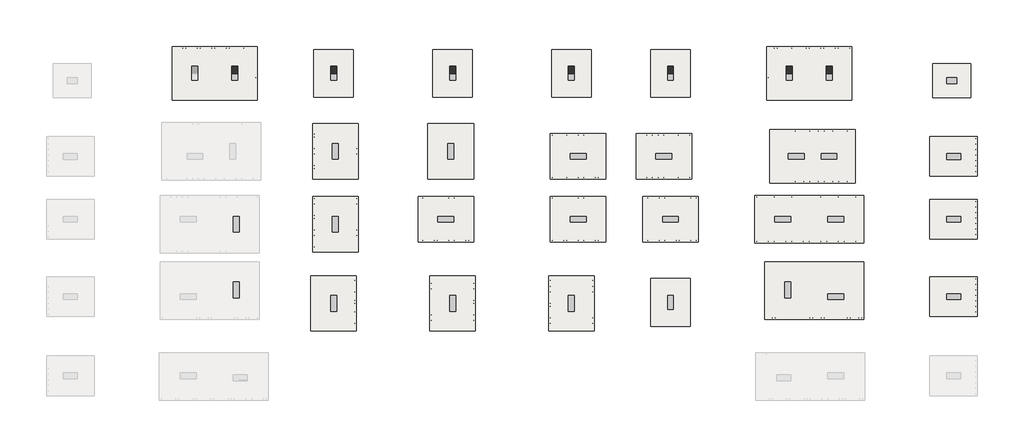
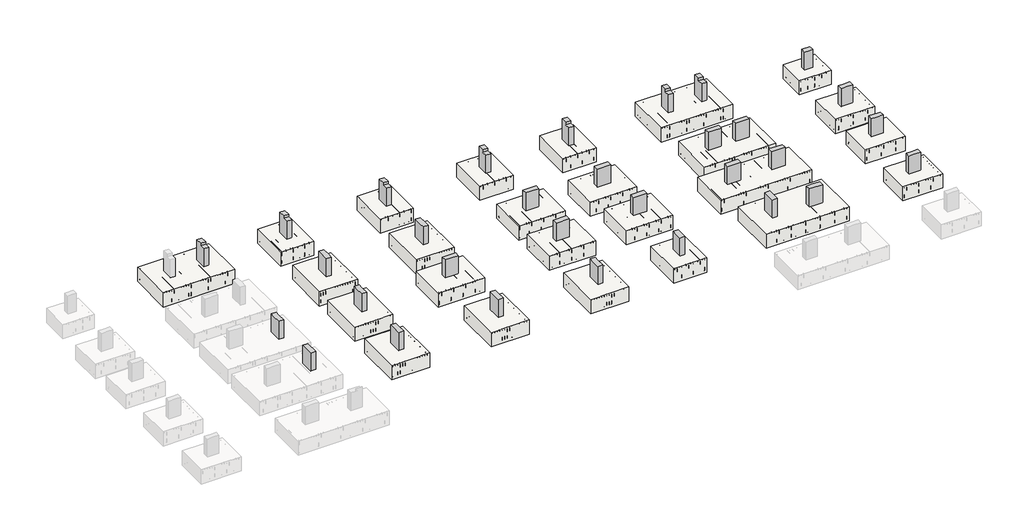
# One storey, part 2 of 21: 31 columns, 25 slabs.
"""IFC4 building model written with IfcOpenShell, lengths in millimetres."""

from ifc_helpers import new_model, si_unit, frame, origin, place, context, project, spatial, polyline, outline, extrude, faceted_brep, transform, mapped, element, save
from components import m_footing_rectangular_1900x1700x900_f1_617558a1, m_footing_rectangular_2300x2800x900_f3_c46bdd4c, m_footing_rectangular_2400x2000x900_f2_ceb4d106, m_footing_rectangular_2700x4300x900_f4_c3563192, m_footing_rectangular_5000x2900x900_f5_2a8e231f, m_footing_rectangular_5500x2400x900_f6_6a8cdcd2

model = new_model("IFC4")

# Units and contexts
model_context = context("Model", 3, world=origin())
ifc_project = project(units=[si_unit("LENGTHUNIT", "METRE", prefix="MILLI")], contexts=[model_context])

# Site, building, storey
site = spatial("IfcSite", under=ifc_project)
building = spatial("IfcBuilding", under=site)
storey = spatial("IfcBuildingStorey", under=building, Elevation=-1100.0)

# Columns
placement = place(None, origin())
element("IfcColumn", 1, ObjectType="M_Concrete-Rectangular-Column : 300X500 C1", at=placement, inside=storey, context=model_context, shape_type="Brep", body=[
    faceted_brep([(20029.1673137, 14604.1704288, -1100.0), (20529.1673137, 14604.1704288, -1100.0), (20529.1673137, 14304.1704288, -1100.0), (20029.1673137, 14304.1704288, -1100.0), (20029.1673137, 14604.1704288, 50.0), (20529.1673137, 14604.1704288, 50.0), (20529.1673137, 14304.1704288, 50.0), (20329.1673137, 14304.1704288, 50.0), (20029.1673137, 14304.1704288, 50.0)], [[[0, 1, 2, 3]], [[1, 0, 4, 5]], [[2, 1, 5, 6]], [[3, 2, 6, 7, 8]], [[0, 3, 8, 4]], [[5, 4, 8, 7, 6]]]),
])
element("IfcColumn", 2, ObjectType="M_Concrete-Rectangular-Column : 300X700 C2", at=placement, inside=storey, context=model_context, shape_type="Brep", body=[
    faceted_brep([(-15760.8326863, 15184.1704288, -1100.0), (-15760.8326863, 14484.1704288, -1100.0), (-16060.8326863, 14484.1704288, -1100.0), (-16060.8326863, 15184.1704288, -1100.0), (-15760.8326863, 15184.1704288, 200.0), (-15760.8326863, 14806.5875097, 200.0), (-15760.8326863, 14806.5875097, 50.0), (-15760.8326863, 14784.1704288, 50.0), (-15760.8326863, 14484.1704288, 50.0), (-15760.8326863, 14484.1704288, -400.0), (-16060.8326863, 14484.1704288, 50.0), (-16060.8326863, 14484.1704288, -400.0), (-16060.8326863, 14784.1704288, 50.0), (-16060.8326863, 14806.5875097, 50.0), (-16060.8326863, 14806.5875097, 200.0), (-16060.8326863, 15184.1704288, 200.0), (-15761.4442233, 14806.5875097, 200.0), (-15761.4442233, 14806.5875097, 50.0)], [[[0, 1, 2, 3]], [[1, 0, 4, 5, 6, 7, 8, 9]], [[2, 1, 9, 8, 10, 11]], [[3, 2, 11, 10, 12, 13, 14, 15]], [[0, 3, 15, 4]], [[4, 15, 14, 16, 5]], [[6, 17, 13, 12, 10, 8, 7]], [[13, 17, 6, 5, 16, 14]]]),
])
element("IfcColumn", 3, ObjectType="M_Concrete-Rectangular-Column : 300X700 C2", at=placement, inside=storey, context=model_context, shape_type="Brep", body=[
    faceted_brep([(-4760.8326863, 15184.1704288, -1100.0), (-4760.8326863, 14484.1704288, -1100.0), (-5060.8326863, 14484.1704288, -1100.0), (-5060.8326863, 15184.1704288, -1100.0), (-4760.8326863, 15184.1704288, 200.0), (-4760.8326863, 14806.5875097, 200.0), (-4760.8326863, 14806.5875097, 50.0), (-4760.8326863, 14784.1704288, 50.0), (-4760.8326863, 14484.1704288, 50.0), (-4760.8326863, 14484.1704288, -400.0), (-5060.8326863, 14484.1704288, 50.0), (-5060.8326863, 14484.1704288, -400.0), (-5060.8326863, 14784.1704288, 50.0), (-5060.8326863, 14806.5875097, 50.0), (-5060.8326863, 14806.5875097, 200.0), (-5060.8326863, 15184.1704288, 200.0)], [[[0, 1, 2, 3]], [[1, 0, 4, 5, 6, 7, 8, 9]], [[2, 1, 9, 8, 10, 11]], [[3, 2, 11, 10, 12, 13, 14, 15]], [[0, 3, 15, 4]], [[4, 15, 14, 5]], [[6, 13, 12, 10, 8, 7]], [[13, 6, 5, 14]]]),
])
element("IfcColumn", 4, ObjectType="M_Concrete-Rectangular-Column : 300X700 C2", at=placement, inside=storey, context=model_context, shape_type="Brep", body=[
    faceted_brep([(1239.1673137, 15184.1704288, -1100.0), (1239.1673137, 14484.1704288, -1100.0), (939.1673137, 14484.1704288, -1100.0), (939.1673137, 15184.1704288, -1100.0), (1239.1673137, 15184.1704288, 200.0), (1239.1673137, 14806.5875097, 200.0), (1239.1673137, 14806.5875097, 50.0), (1239.1673137, 14784.1704288, 50.0), (1239.1673137, 14484.1704288, 50.0), (1239.1673137, 14484.1704288, -400.0), (939.1673137, 14484.1704288, 50.0), (939.1673137, 14484.1704288, -400.0), (939.1673137, 14784.1704288, 50.0), (939.1673137, 14806.5875097, 50.0), (939.1673137, 14806.5875097, 200.0), (939.1673137, 15184.1704288, 200.0)], [[[0, 1, 2, 3]], [[1, 0, 4, 5, 6, 7, 8, 9]], [[2, 1, 9, 8, 10, 11]], [[3, 2, 11, 10, 12, 13, 14, 15]], [[0, 3, 15, 4]], [[4, 15, 14, 5]], [[6, 13, 12, 10, 8, 7]], [[13, 6, 5, 14]]]),
])
element("IfcColumn", 5, ObjectType="M_Concrete-Rectangular-Column : 300X700 C2", at=placement, inside=storey, context=model_context, shape_type="Brep", body=[
    faceted_brep([(6239.1673137, 15184.1301608, -1100.0), (6239.1673137, 14484.1301608, -1100.0), (5939.1673137, 14484.1301608, -1100.0), (5939.1673137, 15184.1301608, -1100.0), (6239.1673137, 15184.1301608, 200.0), (6239.1673137, 14806.5875097, 200.0), (6239.1673137, 14806.5875097, 50.0), (6239.1673137, 14784.1704288, 50.0), (6239.1673137, 14484.1301608, 50.0), (5939.1673137, 14484.1301608, 50.0), (5939.1673137, 14784.1704288, 50.0), (5939.1673137, 14806.5875097, 50.0), (5939.1673137, 14806.5875097, 200.0), (5939.1673137, 15184.1301608, 200.0)], [[[0, 1, 2, 3]], [[1, 0, 4, 5, 6, 7, 8]], [[2, 1, 8, 9]], [[3, 2, 9, 10, 11, 12, 13]], [[0, 3, 13, 4]], [[4, 13, 12, 5]], [[6, 11, 10, 9, 8, 7]], [[11, 6, 5, 12]]]),
])
element("IfcColumn", 6, ObjectType="M_Concrete-Rectangular-Column : 300X700 C2", at=placement, inside=storey, context=model_context, shape_type="Brep", body=[
    faceted_brep([(6239.1673137, 3604.1704288, -1100.0), (6239.1673137, 2904.1704288, -1100.0), (5939.1673137, 2904.1704288, -1100.0), (5939.1673137, 3604.1704288, -1100.0), (6239.1673137, 3604.1704288, 50.0), (6239.1673137, 3276.3054969, 50.0), (6239.1673137, 2904.1704288, 50.0), (5939.1673137, 2904.1704288, 50.0), (5939.1673137, 3304.1704288, 50.0), (5939.1673137, 3604.1704288, 50.0)], [[[0, 1, 2, 3]], [[1, 0, 4, 5, 6]], [[2, 1, 6, 7]], [[3, 2, 7, 8, 9]], [[0, 3, 9, 4]], [[6, 5, 4, 9, 8, 7]]]),
])
element("IfcColumn", 7, ObjectType="M_Concrete-Rectangular-Column : 300X700 C2", at=placement, inside=storey, context=model_context, shape_type="Brep", body=[
    faceted_brep([(12239.1673137, 15184.1704288, -1100.0), (12239.1673137, 14484.1704288, -1100.0), (11939.1673137, 14484.1704288, -1100.0), (11939.1673137, 15184.1704288, -1100.0), (12239.1673137, 15184.1704288, 200.0), (12239.1673137, 14806.5875097, 200.0), (12239.1673137, 14806.5875097, 50.0), (12239.1673137, 14784.1704288, 50.0), (12239.1673137, 14484.1704288, 50.0), (12239.1673137, 14484.1704288, -400.0), (11939.1673137, 14484.1704288, 50.0), (11939.1673137, 14484.1704288, -400.0), (11939.1673137, 14784.1704288, 50.0), (11939.1673137, 14806.5875097, 50.0), (11939.1673137, 14806.5875097, 200.0), (11939.1673137, 15184.1704288, 200.0)], [[[0, 1, 2, 3]], [[1, 0, 4, 5, 6, 7, 8, 9]], [[2, 1, 9, 8, 10, 11]], [[3, 2, 11, 10, 12, 13, 14, 15]], [[0, 3, 15, 4]], [[4, 15, 14, 5]], [[6, 13, 12, 10, 8, 7]], [[13, 6, 5, 14]]]),
])
element("IfcColumn", 8, ObjectType="M_Concrete-Rectangular-Column : 300X700 C2", at=placement, inside=storey, context=model_context, shape_type="SweptSolid", body=[
    extrude(outline(polyline([(15184.1704288, -1100.0), (14484.1704288, -1100.0), (14484.1704288, 50.0), (14806.5875097, 50.0), (14806.5875097, 200.0), (15184.1704288, 200.0), (15184.1704288, -1100.0)])), frame((13939.1673137, 0.0, 0.0), z_axis=(1.0, 0.0, 0.0), x_axis=(0.0, 1.0, 0.0)), (0.0, 0.0, 1.0), 300.0),
])
element("IfcColumn", 9, ObjectType="M_Concrete-Rectangular-Column : 300X700 C2", at=placement, inside=storey, context=model_context, shape_type="Brep", body=[
    faceted_brep([(20029.1673137, 10779.2254822, -1100.0), (20729.1673137, 10779.2254822, -1100.0), (20729.1673137, 10479.2254822, -1100.0), (20029.1673137, 10479.2254822, -1100.0), (20029.1673137, 10779.2254822, -400.0), (20029.1673137, 10779.2254822, 50.0), (20329.1673137, 10779.2254822, 50.0), (20729.1673137, 10779.2254822, 50.0), (20729.1673137, 10479.2254822, 50.0), (20329.1673137, 10479.2254822, 50.0), (20029.1673137, 10479.2254822, 50.0), (20029.1673137, 10479.2254822, -400.0)], [[[0, 1, 2, 3]], [[1, 0, 4, 5, 6, 7]], [[2, 1, 7, 8]], [[3, 2, 8, 9, 10, 11]], [[0, 3, 11, 10, 5, 4]], [[7, 6, 5, 10, 9, 8]]]),
])
element("IfcColumn", 10, ObjectType="M_Concrete-Rectangular-Column : 300X700 C2", at=placement, inside=storey, context=model_context, shape_type="Brep", body=[
    faceted_brep([(20029.1673137, 7604.1704288, -1100.0), (20729.1673137, 7604.1704288, -1100.0), (20729.1673137, 7304.1704288, -1100.0), (20029.1673137, 7304.1704288, -1100.0), (20029.1673137, 7604.1704288, -400.0), (20029.1673137, 7604.1704288, 50.0), (20329.1673137, 7604.1704288, 50.0), (20729.1673137, 7604.1704288, 50.0), (20729.1673137, 7304.1704288, 50.0), (20329.1673137, 7304.1704288, 50.0), (20029.1673137, 7304.1704288, 50.0), (20029.1673137, 7304.1704288, -400.0)], [[[0, 1, 2, 3]], [[1, 0, 4, 5, 6, 7]], [[2, 1, 7, 8]], [[3, 2, 8, 9, 10, 11]], [[0, 3, 11, 10, 5, 4]], [[7, 6, 5, 10, 9, 8]]]),
])
element("IfcColumn", 11, ObjectType="M_Concrete-Rectangular-Column : 300X700 C2", at=placement, inside=storey, context=model_context, shape_type="Brep", body=[
    faceted_brep([(20029.1673137, 3694.1704288, -1100.0), (20729.1673137, 3694.1704288, -1100.0), (20729.1673137, 3394.1704288, -1100.0), (20029.1673137, 3394.1704288, -1100.0), (20029.1673137, 3694.1704288, -400.0), (20029.1673137, 3694.1704288, 50.0), (20329.1673137, 3694.1704288, 50.0), (20729.1673137, 3694.1704288, 50.0), (20729.1673137, 3394.1704288, 50.0), (20329.1673137, 3394.1704288, 50.0), (20029.1673137, 3394.1704288, 50.0), (20029.1673137, 3394.1704288, -400.0)], [[[0, 1, 2, 3]], [[1, 0, 4, 5, 6, 7]], [[2, 1, 7, 8]], [[3, 2, 8, 9, 10, 11]], [[0, 3, 11, 10, 5, 4]], [[7, 6, 5, 10, 9, 8]]]),
])
element("IfcColumn", 12, ObjectType="M_Concrete-Rectangular-Column : 300X700 C2", at=placement, inside=storey, context=model_context, shape_type="Brep", body=[
    faceted_brep([(-11060.8326863, 14484.1704288, -1100.0), (-11060.8326863, 15184.1704288, -1100.0), (-10760.8326863, 15184.1704288, -1100.0), (-10760.8326863, 14484.1704288, -1100.0), (-11060.8326863, 14484.1704288, -400.0), (-11060.8326863, 14484.1704288, 50.0), (-11060.8326863, 14784.1704288, 50.0), (-11060.8326863, 14806.5875097, 50.0), (-11060.8326863, 14806.5875097, 200.0), (-11060.8326863, 15184.1704288, 200.0), (-10760.8326863, 15184.1704288, 200.0), (-10760.8326863, 14806.5875097, 200.0), (-10760.8326863, 14806.5875097, 50.0), (-10760.8326863, 14784.1704288, 50.0), (-10760.8326863, 14484.1704288, 50.0), (-10760.8326863, 14484.1704288, -400.0)], [[[0, 1, 2, 3]], [[1, 0, 4, 5, 6, 7, 8, 9]], [[2, 1, 9, 10]], [[3, 2, 10, 11, 12, 13, 14, 15]], [[0, 3, 15, 14, 5, 4]], [[10, 9, 8, 11]], [[12, 7, 6, 5, 14, 13]], [[7, 12, 11, 8]]]),
])
element("IfcColumn", 13, ObjectType="M_Concrete-Rectangular-Column : 300X800 C3", at=placement, inside=storey, context=model_context, shape_type="Brep", body=[
    faceted_brep([(-15970.8326863, 6804.1704288, -1100.0), (-15970.8326863, 7604.1704288, -1100.0), (-15670.8326863, 7604.1704288, -1100.0), (-15670.8326863, 6804.1704288, -1100.0), (-15970.8326863, 6804.1704288, 50.0), (-15970.8326863, 7304.1704288, 50.0), (-15970.8326863, 7354.7105431, 50.0), (-15970.8326863, 7604.1704288, 50.0), (-15670.8326863, 7604.1704288, 50.0), (-15670.8326863, 7604.1704288, -400.0), (-15670.8326863, 7304.1704288, 50.0), (-15670.8326863, 6804.1704288, 50.0)], [[[0, 1, 2, 3]], [[1, 0, 4, 5, 6, 7]], [[2, 1, 7, 8, 9]], [[3, 2, 9, 8, 10, 11]], [[0, 3, 11, 4]], [[7, 6, 5, 4, 11, 10, 8]]]),
])
element("IfcColumn", 14, ObjectType="M_Concrete-Rectangular-Column : 300X800 C3", at=placement, inside=storey, context=model_context, shape_type="SweptSolid", body=[
    extrude(outline(polyline([(-15970.8326863, 3484.1704288), (-15970.8326863, 4284.1704288), (-15670.8326863, 4284.1704288), (-15670.8326863, 3484.1704288), (-15970.8326863, 3484.1704288)])), frame((0.0, 0.0, -1100.0), z_axis=(0.0, 0.0, 1.0), x_axis=(1.0, 0.0, 0.0)), (0.0, 0.0, 1.0), 1150.0),
])
element("IfcColumn", 15, ObjectType="M_Concrete-Rectangular-Column : 300X800 C3", at=placement, inside=storey, context=model_context, shape_type="Brep", body=[
    faceted_brep([(-10670.8326863, 11284.1704288, -1100.0), (-10670.8326863, 10484.1704288, -1100.0), (-10970.8326863, 10484.1704288, -1100.0), (-10970.8326863, 11284.1704288, -1100.0), (-10670.8326863, 11284.1704288, 50.0), (-10670.8326863, 10784.1704288, 50.0), (-10670.8326863, 10484.1704288, 50.0), (-10670.8326863, 10484.1704288, -400.0), (-10970.8326863, 10484.1704288, 50.0), (-10970.8326863, 10484.1704288, -400.0), (-10970.8326863, 10784.1704288, 50.0), (-10970.8326863, 11284.1704288, 50.0)], [[[0, 1, 2, 3]], [[1, 0, 4, 5, 6, 7]], [[2, 1, 7, 6, 8, 9]], [[3, 2, 9, 8, 10, 11]], [[0, 3, 11, 4]], [[6, 5, 4, 11, 10, 8]]]),
])
element("IfcColumn", 16, ObjectType="M_Concrete-Rectangular-Column : 300X800 C3", at=placement, inside=storey, context=model_context, shape_type="Brep", body=[
    faceted_brep([(-10670.8326863, 7604.1704288, -1100.0), (-10670.8326863, 6804.1704288, -1100.0), (-10970.8326863, 6804.1704288, -1100.0), (-10970.8326863, 7604.1704288, -1100.0), (-10670.8326863, 7604.1704288, -400.0), (-10670.8326863, 7604.1704288, 50.0), (-10670.8326863, 7350.6221749, 50.0), (-10670.8326863, 6804.1704288, 50.0), (-10970.8326863, 6804.1704288, 50.0), (-10970.8326863, 7304.1704288, 50.0), (-10970.8326863, 7604.1704288, 50.0), (-10970.8326863, 7604.1704288, -400.0)], [[[0, 1, 2, 3]], [[1, 0, 4, 5, 6, 7]], [[2, 1, 7, 8]], [[3, 2, 8, 9, 10, 11]], [[0, 3, 11, 10, 5, 4]], [[7, 6, 5, 10, 9, 8]]]),
])
element("IfcColumn", 17, ObjectType="M_Concrete-Rectangular-Column : 300X800 C3", at=placement, inside=storey, context=model_context, shape_type="Brep", body=[
    faceted_brep([(-4850.8326863, 11284.1704288, -1100.0), (-4850.8326863, 10484.1704288, -1100.0), (-5150.8326863, 10484.1704288, -1100.0), (-5150.8326863, 11284.1704288, -1100.0), (-4850.8326863, 11284.1704288, 50.0), (-4850.8326863, 10784.1704288, 50.0), (-4850.8326863, 10484.1704288, 50.0), (-4850.8326863, 10484.1704288, -400.0), (-5150.8326863, 10484.1704288, 50.0), (-5150.8326863, 10484.1704288, -400.0), (-5150.8326863, 10784.1704288, 50.0), (-5150.8326863, 11284.1704288, 50.0)], [[[0, 1, 2, 3]], [[1, 0, 4, 5, 6, 7]], [[2, 1, 7, 6, 8, 9]], [[3, 2, 9, 8, 10, 11]], [[0, 3, 11, 4]], [[6, 5, 4, 11, 10, 8]]]),
])
element("IfcColumn", 18, ObjectType="M_Concrete-Rectangular-Column : 300X800 C3", at=placement, inside=storey, context=model_context, shape_type="Brep", body=[
    faceted_brep([(-10760.8326863, 3604.1704288, -1100.0), (-10760.8326863, 2804.1704288, -1100.0), (-11060.8326863, 2804.1704288, -1100.0), (-11060.8326863, 3604.1704288, -1100.0), (-10760.8326863, 3604.1704288, 50.0), (-10760.8326863, 3304.1704288, 50.0), (-10760.8326863, 2804.1704288, 50.0), (-11060.8326863, 2804.1704288, 50.0), (-11060.8326863, 3303.9418326, 50.0), (-11060.8326863, 3604.1704288, 50.0)], [[[0, 1, 2, 3]], [[1, 0, 4, 5, 6]], [[2, 1, 6, 7]], [[3, 2, 7, 8, 9]], [[0, 3, 9, 4]], [[6, 5, 4, 9, 8, 7]]]),
])
element("IfcColumn", 19, ObjectType="M_Concrete-Rectangular-Column : 300X800 C3", at=placement, inside=storey, context=model_context, shape_type="Brep", body=[
    faceted_brep([(-4760.8326863, 3604.1704288, -1100.0), (-4760.8326863, 2804.1704288, -1100.0), (-5060.8326863, 2804.1704288, -1100.0), (-5060.8326863, 3604.1704288, -1100.0), (-4760.8326863, 3604.1704288, -400.0), (-4760.8326863, 3604.1704288, 50.0), (-4760.8326863, 3304.1704288, 50.0), (-4760.8326863, 2804.1704288, 50.0), (-5060.8326863, 2804.1704288, 50.0), (-5060.8326863, 3304.1704288, 50.0), (-5060.8326863, 3604.1704288, 50.0), (-5060.8326863, 3604.1704288, -400.0)], [[[0, 1, 2, 3]], [[1, 0, 4, 5, 6, 7]], [[2, 1, 7, 8]], [[3, 2, 8, 9, 10, 11]], [[0, 3, 11, 10, 5, 4]], [[7, 6, 5, 10, 9, 8]]]),
])
element("IfcColumn", 20, ObjectType="M_Concrete-Rectangular-Column : 300X800 C3", at=placement, inside=storey, context=model_context, shape_type="Brep", body=[
    faceted_brep([(-5650.8326863, 7604.1704288, -1100.0), (-4850.8326863, 7604.1704288, -1100.0), (-4850.8326863, 7304.1704288, -1100.0), (-5650.8326863, 7304.1704288, -1100.0), (-5650.8326863, 7604.1704288, -400.0), (-5650.8326863, 7604.1704288, 50.0), (-4850.8326863, 7604.1704288, 50.0), (-4850.8326863, 7604.1704288, -400.0), (-4850.8326863, 7304.1704288, 50.0), (-4850.8326863, 7304.1704288, -400.0), (-5650.8326863, 7304.1704288, 50.0), (-5650.8326863, 7304.1704288, -400.0)], [[[0, 1, 2, 3]], [[1, 0, 4, 5, 6, 7]], [[2, 1, 7, 6, 8, 9]], [[3, 2, 9, 8, 10, 11]], [[0, 3, 11, 10, 5, 4]], [[6, 5, 10, 8]]]),
])
element("IfcColumn", 21, ObjectType="M_Concrete-Rectangular-Column : 300X800 C3", at=placement, inside=storey, context=model_context, shape_type="Brep", body=[
    faceted_brep([(1029.1673137, 10784.1704288, -1100.0), (1829.1673137, 10784.1704288, -1100.0), (1829.1673137, 10484.1704288, -1100.0), (1029.1673137, 10484.1704288, -1100.0), (1029.1673137, 10784.1704288, -400.0), (1029.1673137, 10784.1704288, 50.0), (1829.1673137, 10784.1704288, 50.0), (1829.1673137, 10784.1704288, -400.0), (1829.1673137, 10484.1704288, 50.0), (1829.1673137, 10484.1704288, -400.0), (1029.1673137, 10484.1704288, 50.0), (1029.1673137, 10484.1704288, -400.0)], [[[0, 1, 2, 3]], [[1, 0, 4, 5, 6, 7]], [[2, 1, 7, 6, 8, 9]], [[3, 2, 9, 8, 10, 11]], [[0, 3, 11, 10, 5, 4]], [[6, 5, 10, 8]]]),
])
element("IfcColumn", 22, ObjectType="M_Concrete-Rectangular-Column : 300X800 C3", at=placement, inside=storey, context=model_context, shape_type="Brep", body=[
    faceted_brep([(5349.1673137, 10784.1704288, -1100.0), (6149.1673137, 10784.1704288, -1100.0), (6149.1673137, 10484.1704288, -1100.0), (5349.1673137, 10484.1704288, -1100.0), (5349.1673137, 10784.1704288, -400.0), (5349.1673137, 10784.1704288, 50.0), (6149.1673137, 10784.1704288, 50.0), (6149.1673137, 10784.1704288, -400.0), (6149.1673137, 10634.1704288, 50.0), (6149.1673137, 10484.1704288, 50.0), (5349.1673137, 10484.1704288, 50.0), (5349.1673137, 10484.1704288, -400.0)], [[[0, 1, 2, 3]], [[1, 0, 4, 5, 6, 7]], [[2, 1, 7, 6, 8, 9]], [[3, 2, 9, 10, 11]], [[0, 3, 11, 10, 5, 4]], [[6, 5, 10, 9, 8]]]),
])
element("IfcColumn", 23, ObjectType="M_Concrete-Rectangular-Column : 300X800 C3", at=placement, inside=storey, context=model_context, shape_type="Brep", body=[
    faceted_brep([(5689.1673137, 7604.1704288, -1100.0), (6489.1673137, 7604.1704288, -1100.0), (6489.1673137, 7304.1704288, -1100.0), (5689.1673137, 7304.1704288, -1100.0), (5689.1673137, 7604.1704288, -400.0), (5689.1673137, 7604.1704288, 50.0), (6489.1673137, 7604.1704288, 50.0), (6489.1673137, 7604.1704288, -400.0), (6489.1673137, 7304.1704288, 50.0), (6489.1673137, 7304.1704288, -400.0), (5689.1673137, 7304.1704288, 50.0), (5689.1673137, 7304.1704288, -400.0)], [[[0, 1, 2, 3]], [[1, 0, 4, 5, 6, 7]], [[2, 1, 7, 6, 8, 9]], [[3, 2, 9, 8, 10, 11]], [[0, 3, 11, 10, 5, 4]], [[6, 5, 10, 8]]]),
])
element("IfcColumn", 24, ObjectType="M_Concrete-Rectangular-Column : 300X800 C3", at=placement, inside=storey, context=model_context, shape_type="Brep", body=[
    faceted_brep([(1029.1673137, 7604.1704288, -1100.0), (1829.1673137, 7604.1704288, -1100.0), (1829.1673137, 7304.1704288, -1100.0), (1029.1673137, 7304.1704288, -1100.0), (1029.1673137, 7604.1704288, 50.0), (1829.1673137, 7604.1704288, 50.0), (1829.1673137, 7604.1704288, -400.0), (1829.1673137, 7304.1704288, 50.0), (1829.1673137, 7304.1704288, -400.0), (1029.1673137, 7304.1704288, 50.0)], [[[0, 1, 2, 3]], [[1, 0, 4, 5, 6]], [[2, 1, 6, 5, 7, 8]], [[3, 2, 8, 7, 9]], [[0, 3, 9, 4]], [[5, 4, 9, 7]]]),
])
element("IfcColumn", 25, ObjectType="M_Concrete-Rectangular-Column : 300X800 C3", at=placement, inside=storey, context=model_context, shape_type="Brep", body=[
    faceted_brep([(939.1673137, 2804.1704288, -1100.0), (939.1673137, 3604.1704288, -1100.0), (1239.1673137, 3604.1704288, -1100.0), (1239.1673137, 2804.1704288, -1100.0), (939.1673137, 2804.1704288, 50.0), (939.1673137, 3304.1704288, 50.0), (939.1673137, 3604.1704288, 50.0), (939.1673137, 3604.1704288, -400.0), (1239.1673137, 3604.1704288, 50.0), (1239.1673137, 3604.1704288, -400.0), (1239.1673137, 3304.1704288, 50.0), (1239.1673137, 2804.1704288, 50.0)], [[[0, 1, 2, 3]], [[1, 0, 4, 5, 6, 7]], [[2, 1, 7, 6, 8, 9]], [[3, 2, 9, 8, 10, 11]], [[0, 3, 11, 4]], [[6, 5, 4, 11, 10, 8]]]),
])
element("IfcColumn", 26, ObjectType="M_Concrete-Rectangular-Column : 300X800 C3", at=placement, inside=storey, context=model_context, shape_type="Brep", body=[
    faceted_brep([(13689.1673137, 10784.1704288, -1100.0), (14489.1673137, 10784.1704288, -1100.0), (14489.1673137, 10484.1704288, -1100.0), (13689.1673137, 10484.1704288, -1100.0), (13689.1673137, 10784.1704288, -400.0), (13689.1673137, 10784.1704288, 50.0), (14489.1673137, 10784.1704288, 50.0), (14489.1673137, 10784.1704288, -400.0), (14489.1673137, 10484.1704288, 50.0), (14489.1673137, 10484.1704288, -400.0), (13689.1673137, 10484.1704288, 50.0), (13689.1673137, 10484.1704288, -400.0)], [[[0, 1, 2, 3]], [[1, 0, 4, 5, 6, 7]], [[2, 1, 7, 6, 8, 9]], [[3, 2, 9, 8, 10, 11]], [[0, 3, 11, 10, 5, 4]], [[6, 5, 10, 8]]]),
])
element("IfcColumn", 27, ObjectType="M_Concrete-Rectangular-Column : 300X800 C3", at=placement, inside=storey, context=model_context, shape_type="Brep", body=[
    faceted_brep([(12029.1673137, 10784.1704288, -1100.0), (12829.1673137, 10784.1704288, -1100.0), (12829.1673137, 10484.1704288, -1100.0), (12029.1673137, 10484.1704288, -1100.0), (12029.1673137, 10784.1704288, -400.0), (12029.1673137, 10784.1704288, 50.0), (12829.1673137, 10784.1704288, 50.0), (12829.1673137, 10784.1704288, -400.0), (12829.1673137, 10484.1704288, 50.0), (12829.1673137, 10484.1704288, -400.0), (12029.1673137, 10484.1704288, 50.0), (12029.1673137, 10484.1704288, -400.0)], [[[0, 1, 2, 3]], [[1, 0, 4, 5, 6, 7]], [[2, 1, 7, 6, 8, 9]], [[3, 2, 9, 8, 10, 11]], [[0, 3, 11, 10, 5, 4]], [[6, 5, 10, 8]]]),
])
element("IfcColumn", 28, ObjectType="M_Concrete-Rectangular-Column : 300X800 C3", at=placement, inside=storey, context=model_context, shape_type="Brep", body=[
    faceted_brep([(11349.1673137, 7604.1704288, -1100.0), (12149.1673137, 7604.1704288, -1100.0), (12149.1673137, 7304.1704288, -1100.0), (11349.1673137, 7304.1704288, -1100.0), (11349.1673137, 7604.1704288, -400.0), (11349.1673137, 7604.1704288, 50.0), (12149.1673137, 7604.1704288, 50.0), (12149.1673137, 7604.1704288, -400.0), (12149.1673137, 7304.1704288, 50.0), (12149.1673137, 7304.1704288, -400.0), (11349.1673137, 7304.1704288, 50.0), (11349.1673137, 7304.1704288, -400.0)], [[[0, 1, 2, 3]], [[1, 0, 4, 5, 6, 7]], [[2, 1, 7, 6, 8, 9]], [[3, 2, 9, 8, 10, 11]], [[0, 3, 11, 10, 5, 4]], [[6, 5, 10, 8]]]),
])
element("IfcColumn", 29, ObjectType="M_Concrete-Rectangular-Column : 300X800 C3", at=placement, inside=storey, context=model_context, shape_type="Brep", body=[
    faceted_brep([(14029.1673137, 7604.1704288, -1100.0), (14829.1673137, 7604.1704288, -1100.0), (14829.1673137, 7304.1704288, -1100.0), (14029.1673137, 7304.1704288, -1100.0), (14029.1673137, 7604.1704288, -400.0), (14029.1673137, 7604.1704288, 50.0), (14829.1673137, 7604.1704288, 50.0), (14829.1673137, 7604.1704288, -400.0), (14829.1673137, 7304.1704288, 50.0), (14829.1673137, 7304.1704288, -400.0), (14029.1673137, 7304.1704288, 50.0), (14029.1673137, 7304.1704288, -400.0)], [[[0, 1, 2, 3]], [[1, 0, 4, 5, 6, 7]], [[2, 1, 7, 6, 8, 9]], [[3, 2, 9, 8, 10, 11]], [[0, 3, 11, 10, 5, 4]], [[6, 5, 10, 8]]]),
])
element("IfcColumn", 30, ObjectType="M_Concrete-Rectangular-Column : 300X800 C3", at=placement, inside=storey, context=model_context, shape_type="Brep", body=[
    faceted_brep([(14029.1673137, 3694.1704288, -1100.0), (14829.1673137, 3694.1704288, -1100.0), (14829.1673137, 3394.1704288, -1100.0), (14029.1673137, 3394.1704288, -1100.0), (14029.1673137, 3694.1704288, -400.0), (14029.1673137, 3694.1704288, 50.0), (14329.1673137, 3694.1704288, 50.0), (14829.1673137, 3694.1704288, 50.0), (14829.1673137, 3394.1704288, 50.0), (14329.1673137, 3394.1704288, 50.0), (14029.1673137, 3394.1704288, 50.0), (14029.1673137, 3394.1704288, -400.0)], [[[0, 1, 2, 3]], [[1, 0, 4, 5, 6, 7]], [[2, 1, 7, 8]], [[3, 2, 8, 9, 10, 11]], [[0, 3, 11, 10, 5, 4]], [[7, 6, 5, 10, 9, 8]]]),
])
element("IfcColumn", 31, ObjectType="M_Concrete-Rectangular-Column : 300X800 C3", at=placement, inside=storey, context=model_context, shape_type="SweptSolid", body=[
    extrude(outline(polyline([(11849.1673137, 3484.1704288), (11849.1673137, 4284.1704288), (12149.1673137, 4284.1704288), (12149.1673137, 3484.1704288), (11849.1673137, 3484.1704288)])), frame((0.0, 0.0, -1100.0), z_axis=(0.0, 0.0, 1.0), x_axis=(1.0, 0.0, 0.0)), (0.0, 0.0, 1.0), 1150.0),
])

# Slabs
m_footing_rectangular_1900x1700x900_f1_shape = m_footing_rectangular_1900x1700x900_f1_617558a1(model_context)
element("IfcSlab", 32, ObjectType="M_Footing-Rectangular : 1900X1700X900 F1", at=placement, inside=storey, context=model_context, shape_type="MappedRepresentation", body=[
    mapped(m_footing_rectangular_1900x1700x900_f1_shape, transform((20279.1673137, 14454.1704288, -1100.0), x_axis=(1.0, 0.0, 0.0), y_axis=(0.0, 1.0, 0.0), z_axis=(0.0, 0.0, 1.0))),
])
m_footing_rectangular_2300x2800x900_f3_shape = m_footing_rectangular_2300x2800x900_f3_c46bdd4c(model_context)
element("IfcSlab", 33, ObjectType="M_Footing-Rectangular : 2300X2800X900 F3", at=placement, inside=storey, context=model_context, shape_type="MappedRepresentation", body=[
    mapped(m_footing_rectangular_2300x2800x900_f3_shape, transform((-10820.8326863, 10884.1704288, -1100.0), x_axis=(1.0, 0.0, 0.0), y_axis=(0.0, 1.0, 0.0), z_axis=(0.0, 0.0, 1.0))),
])
element("IfcSlab", 34, ObjectType="M_Footing-Rectangular : 2300X2800X900 F3", at=placement, inside=storey, context=model_context, shape_type="MappedRepresentation", body=[
    mapped(m_footing_rectangular_2300x2800x900_f3_shape, transform((-5000.8326863, 10884.1704288, -1100.0), x_axis=(1.0, 0.0, 0.0), y_axis=(0.0, 1.0, 0.0), z_axis=(0.0, 0.0, 1.0))),
])
element("IfcSlab", 35, ObjectType="M_Footing-Rectangular : 2300X2800X900 F3", at=placement, inside=storey, context=model_context, shape_type="MappedRepresentation", body=[
    mapped(m_footing_rectangular_2300x2800x900_f3_shape, transform((-10820.8326863, 7204.1704288, -1100.0), x_axis=(1.0, 0.0, 0.0), y_axis=(0.0, 1.0, 0.0), z_axis=(0.0, 0.0, 1.0))),
])
element("IfcSlab", 36, ObjectType="M_Footing-Rectangular : 2300X2800X900 F3", at=placement, inside=storey, context=model_context, shape_type="MappedRepresentation", body=[
    mapped(m_footing_rectangular_2300x2800x900_f3_shape, transform((-10910.8326863, 3204.1704288, -1100.0), x_axis=(1.0, 0.0, 0.0), y_axis=(0.0, 1.0, 0.0), z_axis=(0.0, 0.0, 1.0))),
])
element("IfcSlab", 37, ObjectType="M_Footing-Rectangular : 2300X2800X900 F3", at=placement, inside=storey, context=model_context, shape_type="MappedRepresentation", body=[
    mapped(m_footing_rectangular_2300x2800x900_f3_shape, transform((-4910.8326863, 3204.1704288, -1100.0), x_axis=(1.0, 0.0, 0.0), y_axis=(0.0, 1.0, 0.0), z_axis=(0.0, 0.0, 1.0))),
])
element("IfcSlab", 38, ObjectType="M_Footing-Rectangular : 2300X2800X900 F3", at=placement, inside=storey, context=model_context, shape_type="MappedRepresentation", body=[
    mapped(m_footing_rectangular_2300x2800x900_f3_shape, transform((-5250.8326863, 7454.1704288, -1100.0), x_axis=(0.0, 1.0, 0.0), y_axis=(-1.0, 0.0, 0.0), z_axis=(0.0, 0.0, 1.0))),
])
element("IfcSlab", 39, ObjectType="M_Footing-Rectangular : 2300X2800X900 F3", at=placement, inside=storey, context=model_context, shape_type="MappedRepresentation", body=[
    mapped(m_footing_rectangular_2300x2800x900_f3_shape, transform((1429.1673137, 10634.1704288, -1100.0), x_axis=(0.0, 1.0, 0.0), y_axis=(-1.0, 0.0, 0.0), z_axis=(0.0, 0.0, 1.0))),
])
element("IfcSlab", 40, ObjectType="M_Footing-Rectangular : 2300X2800X900 F3", at=placement, inside=storey, context=model_context, shape_type="MappedRepresentation", body=[
    mapped(m_footing_rectangular_2300x2800x900_f3_shape, transform((1429.1673137, 7454.1704288, -1100.0), x_axis=(0.0, 1.0, 0.0), y_axis=(-1.0, 0.0, 0.0), z_axis=(0.0, 0.0, 1.0))),
])
element("IfcSlab", 41, ObjectType="M_Footing-Rectangular : 2300X2800X900 F3", at=placement, inside=storey, context=model_context, shape_type="MappedRepresentation", body=[
    mapped(m_footing_rectangular_2300x2800x900_f3_shape, transform((1089.1673137, 3204.1704288, -1100.0), x_axis=(-1.0, 0.0, 0.0), y_axis=(0.0, -1.0, 0.0), z_axis=(0.0, 0.0, 1.0))),
])
element("IfcSlab", 42, ObjectType="M_Footing-Rectangular : 2300X2800X900 F3", at=placement, inside=storey, context=model_context, shape_type="MappedRepresentation", body=[
    mapped(m_footing_rectangular_2300x2800x900_f3_shape, transform((6089.1673137, 7454.1704288, -1100.0), x_axis=(0.0, -1.0, 0.0), y_axis=(1.0, 0.0, 0.0), z_axis=(0.0, 0.0, 1.0))),
])
element("IfcSlab", 43, ObjectType="M_Footing-Rectangular : 2300X2800X900 F3", at=placement, inside=storey, context=model_context, shape_type="MappedRepresentation", body=[
    mapped(m_footing_rectangular_2300x2800x900_f3_shape, transform((5749.1673137, 10634.1704288, -1100.0), x_axis=(0.0, -1.0, 0.0), y_axis=(1.0, 0.0, 0.0), z_axis=(0.0, 0.0, 1.0))),
])
m_footing_rectangular_2400x2000x900_f2_shape = m_footing_rectangular_2400x2000x900_f2_ceb4d106(model_context)
element("IfcSlab", 44, ObjectType="M_Footing-Rectangular : 2400X2000X900 F2", at=placement, inside=storey, context=model_context, shape_type="MappedRepresentation", body=[
    mapped(m_footing_rectangular_2400x2000x900_f2_shape, transform((-10910.8326863, 14834.170481, -1100.0), x_axis=(0.0, 1.0, 0.0), y_axis=(-1.0, 0.0, 0.0), z_axis=(0.0, 0.0, 1.0))),
])
element("IfcSlab", 45, ObjectType="M_Footing-Rectangular : 2400X2000X900 F2", at=placement, inside=storey, context=model_context, shape_type="MappedRepresentation", body=[
    mapped(m_footing_rectangular_2400x2000x900_f2_shape, transform((-4910.8326863, 14834.170481, -1100.0), x_axis=(0.0, 1.0, 0.0), y_axis=(-1.0, 0.0, 0.0), z_axis=(0.0, 0.0, 1.0))),
])
element("IfcSlab", 46, ObjectType="M_Footing-Rectangular : 2400X2000X900 F2", at=placement, inside=storey, context=model_context, shape_type="MappedRepresentation", body=[
    mapped(m_footing_rectangular_2400x2000x900_f2_shape, transform((1089.1673137, 14834.170481, -1100.0), x_axis=(0.0, 1.0, 0.0), y_axis=(-1.0, 0.0, 0.0), z_axis=(0.0, 0.0, 1.0))),
])
element("IfcSlab", 47, ObjectType="M_Footing-Rectangular : 2400X2000X900 F2", at=placement, inside=storey, context=model_context, shape_type="MappedRepresentation", body=[
    mapped(m_footing_rectangular_2400x2000x900_f2_shape, transform((6089.1673137, 14833.8679953, -1100.0), x_axis=(0.0, 1.0, 0.0), y_axis=(-1.0, 0.0, 0.0), z_axis=(0.0, 0.0, 1.0))),
])
element("IfcSlab", 48, ObjectType="M_Footing-Rectangular : 2400X2000X900 F2", at=placement, inside=storey, context=model_context, shape_type="MappedRepresentation", body=[
    mapped(m_footing_rectangular_2400x2000x900_f2_shape, transform((6089.1673137, 3253.8679953, -1100.0), x_axis=(0.0, 1.0, 0.0), y_axis=(-1.0, 0.0, 0.0), z_axis=(0.0, 0.0, 1.0))),
])
element("IfcSlab", 49, ObjectType="M_Footing-Rectangular : 2400X2000X900 F2", at=placement, inside=storey, context=model_context, shape_type="MappedRepresentation", body=[
    mapped(m_footing_rectangular_2400x2000x900_f2_shape, transform((20379.1673659, 10629.2254822, -1100.0), x_axis=(-1.0, 0.0, 0.0), y_axis=(0.0, -1.0, 0.0), z_axis=(0.0, 0.0, 1.0))),
])
element("IfcSlab", 50, ObjectType="M_Footing-Rectangular : 2400X2000X900 F2", at=placement, inside=storey, context=model_context, shape_type="MappedRepresentation", body=[
    mapped(m_footing_rectangular_2400x2000x900_f2_shape, transform((20379.1673659, 7454.1704288, -1100.0), x_axis=(-1.0, 0.0, 0.0), y_axis=(0.0, -1.0, 0.0), z_axis=(0.0, 0.0, 1.0))),
])
element("IfcSlab", 51, ObjectType="M_Footing-Rectangular : 2400X2000X900 F2", at=placement, inside=storey, context=model_context, shape_type="MappedRepresentation", body=[
    mapped(m_footing_rectangular_2400x2000x900_f2_shape, transform((20379.1673659, 3544.1704288, -1100.0), x_axis=(-1.0, 0.0, 0.0), y_axis=(0.0, -1.0, 0.0), z_axis=(0.0, 0.0, 1.0))),
])
m_footing_rectangular_2700x4300x900_f4_shape = m_footing_rectangular_2700x4300x900_f4_c3563192(model_context)
element("IfcSlab", 52, ObjectType="M_Footing-Rectangular : 2700X4300X900 F4", at=placement, inside=storey, context=model_context, shape_type="MappedRepresentation", body=[
    mapped(m_footing_rectangular_2700x4300x900_f4_shape, transform((-16910.8326863, 14834.1704288, -1100.0), x_axis=(0.0, 1.0, 0.0), y_axis=(-1.0, 0.0, 0.0), z_axis=(0.0, 0.0, 1.0))),
])
element("IfcSlab", 53, ObjectType="M_Footing-Rectangular : 2700X4300X900 F4", at=placement, inside=storey, context=model_context, shape_type="MappedRepresentation", body=[
    mapped(m_footing_rectangular_2700x4300x900_f4_shape, transform((13259.1673137, 10634.1704288, -1100.0), x_axis=(0.0, 1.0, 0.0), y_axis=(-1.0, 0.0, 0.0), z_axis=(0.0, 0.0, 1.0))),
])
element("IfcSlab", 54, ObjectType="M_Footing-Rectangular : 2700X4300X900 F4", at=placement, inside=storey, context=model_context, shape_type="MappedRepresentation", body=[
    mapped(m_footing_rectangular_2700x4300x900_f4_shape, transform((13089.1673137, 14834.1704288, -1100.0), x_axis=(0.0, 1.0, 0.0), y_axis=(-1.0, 0.0, 0.0), z_axis=(0.0, 0.0, 1.0))),
])
m_footing_rectangular_5000x2900x900_f5_shape = m_footing_rectangular_5000x2900x900_f5_2a8e231f(model_context)
element("IfcSlab", 55, ObjectType="M_Footing-Rectangular : 5000X2900X900 F5", at=placement, inside=storey, context=model_context, shape_type="MappedRepresentation", body=[
    mapped(m_footing_rectangular_5000x2900x900_f5_shape, transform((13339.1673137, 3839.1704288, -1100.0), x_axis=(0.0, 1.0, 0.0), y_axis=(-1.0, 0.0, 0.0), z_axis=(0.0, 0.0, 1.0))),
])
m_footing_rectangular_5500x2400x900_f6_shape = m_footing_rectangular_5500x2400x900_f6_6a8cdcd2(model_context)
element("IfcSlab", 56, ObjectType="M_Footing-Rectangular : 5500X2400X900 F6", at=placement, inside=storey, context=model_context, shape_type="MappedRepresentation", body=[
    mapped(m_footing_rectangular_5500x2400x900_f6_shape, transform((13089.1673137, 7454.1704288, -1100.0), x_axis=(0.0, 1.0, 0.0), y_axis=(-1.0, 0.0, 0.0), z_axis=(0.0, 0.0, 1.0))),
])

save(model, "model.ifc")

# Revit data of these elements
# Type "M_Concrete-Rectangular-Column : 300X500 C1"
#   b = 300 mm
#   h = 500 mm
#   Structural Material [instance default] = Concrete, Cast-in-Place gray
# Type "M_Concrete-Rectangular-Column : 300X700 C2"
#   b = 300 mm
#   h = 700 mm
#   Structural Material [instance default] = Concrete, Cast-in-Place gray
# Type "M_Concrete-Rectangular-Column : 300X800 C3"
#   b = 300 mm
#   h = 800 mm
#   Structural Material [instance default] = Concrete, Cast-in-Place gray
# Type "M_Footing-Rectangular : 1900X1700X900 F1"
#   Width = 1900 mm
#   Length = 1700 mm
#   Foundation Thickness = 900 mm
#   Structural Material [instance default] = Concrete, Cast-in-Place gray
#   Assembly Code = ""
# Type "M_Footing-Rectangular : 2300X2800X900 F3"
#   Width = 2300 mm
#   Length = 2800 mm
#   Foundation Thickness = 900 mm
#   Structural Material [instance default] = Concrete, Cast-in-Place gray
#   Assembly Code = ""
# Type "M_Footing-Rectangular : 2400X2000X900 F2"
#   Width = 2400 mm
#   Length = 2000 mm
#   Foundation Thickness = 900 mm
#   Structural Material [instance default] = Concrete, Cast-in-Place gray
#   Assembly Code = ""
# Type "M_Footing-Rectangular : 2700X4300X900 F4"
#   Width = 2700 mm
#   Length = 4300 mm
#   Foundation Thickness = 900 mm
#   Structural Material [instance default] = Concrete, Cast-in-Place gray
#   Assembly Code = ""
# Type "M_Footing-Rectangular : 5000X2900X900 F5"
#   Width = 2900 mm
#   Length = 5000 mm
#   Foundation Thickness = 900 mm
#   Structural Material [instance default] = Concrete, Cast-in-Place gray
#   Assembly Code = ""
# Type "M_Footing-Rectangular : 5500X2400X900 F6"
#   Width = 2400 mm
#   Length = 5500 mm
#   Foundation Thickness = 900 mm
#   Structural Material [instance default] = Concrete, Cast-in-Place gray
#   Assembly Code = ""
# Element 1 (IfcColumn, "M_Concrete-Rectangular-Column : 300X500 C1")
#   Structural Material = Concrete, Cast In Situ
#   Phase Created = New Construction
#   Materials on its faces: "Concrete, Cast In Situ"
# Elements 2, 3, 4, 5, 6, 7, 8, 9, 10, 11, 12 (IfcColumn, "M_Concrete-Rectangular-Column : 300X700 C2")
#   Structural Material = Concrete, Cast In Situ
#   Phase Created = New Construction
#   Materials on its faces: "Concrete, Cast In Situ"
# Elements 13, 14, 15, 16, 17, 18, 19, 20, 21, 22, 23, 24, 25, 26, 27, 28, 29, 30, 31 (IfcColumn, "M_Concrete-Rectangular-Column : 300X800 C3")
#   Structural Material = Concrete, Cast In Situ
#   Phase Created = New Construction
#   Materials on its faces: "Concrete, Cast In Situ"
# Element 32 (IfcSlab, "M_Footing-Rectangular : 1900X1700X900 F1")
#   Structural Material = Concrete, Cast In Situ
#   Phase Created = New Construction
#   Materials on its faces: "Concrete, Cast In Situ"
# Elements 33, 34, 35, 36, 37, 38, 39, 40, 41, 42, 43 (IfcSlab, "M_Footing-Rectangular : 2300X2800X900 F3")
#   Structural Material = Concrete, Cast In Situ
#   Phase Created = New Construction
#   Materials on its faces: "Concrete, Cast In Situ"
# Elements 44, 45, 46, 47, 48, 49, 50, 51 (IfcSlab, "M_Footing-Rectangular : 2400X2000X900 F2")
#   Structural Material = Concrete, Cast In Situ
#   Phase Created = New Construction
#   Materials on its faces: "Concrete, Cast In Situ"
# Elements 52, 53, 54 (IfcSlab, "M_Footing-Rectangular : 2700X4300X900 F4")
#   Structural Material = Concrete, Cast In Situ
#   Phase Created = New Construction
#   Materials on its faces: "Concrete, Cast In Situ"
# Element 55 (IfcSlab, "M_Footing-Rectangular : 5000X2900X900 F5")
#   Structural Material = Concrete, Cast In Situ
#   Phase Created = New Construction
#   Materials on its faces: "Concrete, Cast In Situ"
# Element 56 (IfcSlab, "M_Footing-Rectangular : 5500X2400X900 F6")
#   Structural Material = Concrete, Cast In Situ
#   Phase Created = New Construction
#   Materials on its faces: "Concrete, Cast In Situ"
# Materials
#   "Concrete, Cast-in-Place gray": class "Concrete", colour RGB 192 192 192, transparency 0, Description = "Cast-in-place concrete", Cost = 0
#   "Concrete, Cast In Situ": class "Concrete", colour RGB 192 192 192, transparency 0, Description = "physical material", Cost = 0
